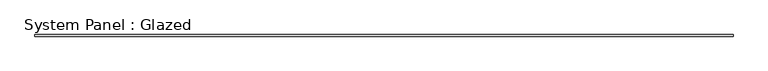
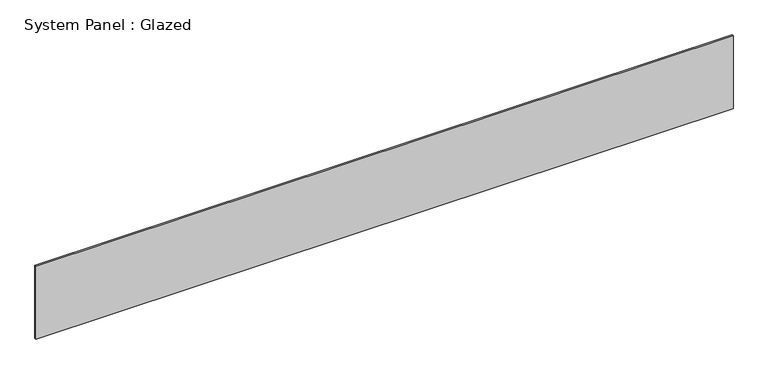
"""IFC4 building model written with IfcOpenShell, lengths in millimetres: plate geometry, System Panel : Glazed."""

from ifc_helpers import new_model, si_unit, origin, origin_with_axes, place, context, project, spatial, polyline, outline, extrude, source, transform, mapped, element, save


def system_panel_glazed_5fdeb3e7(model_context):
    return source(origin(), model_context, "Body", "SweptSolid", [
        extrude(outline(polyline([(5524.5, 19.05), (-5524.5, 19.05), (-5524.5, 44.45), (5524.5, 44.45), (5524.5, 19.05)])), origin_with_axes(), (0.0, 0.0, 1.0), 1219.2),
    ])


if __name__ == "__main__":
    model = new_model("IFC4")
    model_context = context("Model", 3, world=origin())
    ifc_project = project(units=[si_unit("LENGTHUNIT", "METRE", prefix="MILLI")], contexts=[model_context])
    site = spatial("IfcSite", under=ifc_project)
    building = spatial("IfcBuilding", under=site)
    placement = place(None, origin())
    system_panel_glazed_shape = system_panel_glazed_5fdeb3e7(model_context)
    element("IfcPlate", 1, ObjectType="System Panel : Glazed", at=placement, inside=building, context=model_context, shape_type="MappedRepresentation", body=[
        mapped(system_panel_glazed_shape, transform((0.0, 0.0, 0.0), x_axis=(1.0, 0.0, 0.0), y_axis=(0.0, 1.0, 0.0), z_axis=(0.0, 0.0, 1.0))),
    ])
    save(model, "model.ifc")

# Revit data of these elements
# Type "System Panel : Glazed"
#   Construction Type Id = "GSP4R"
#   Analytic Construction = "1/8 in Pilkington single glazing"
#   Visual Light Transmittance = 0.9
#   Solar Heat Gain Coefficient = 0.86
#   Heat Transfer Coefficient (U) = 1.18115 BTU/(h·ft²·°F)
# Element 1 (IfcPlate, "System Panel : Glazed")
#   Materials on its faces: "Glass"
# Materials
#   "Glass": class "Glass", colour RGB 0 128 192, transparency 0.75, Description = "Soda Lime Glass", Cost = 0
